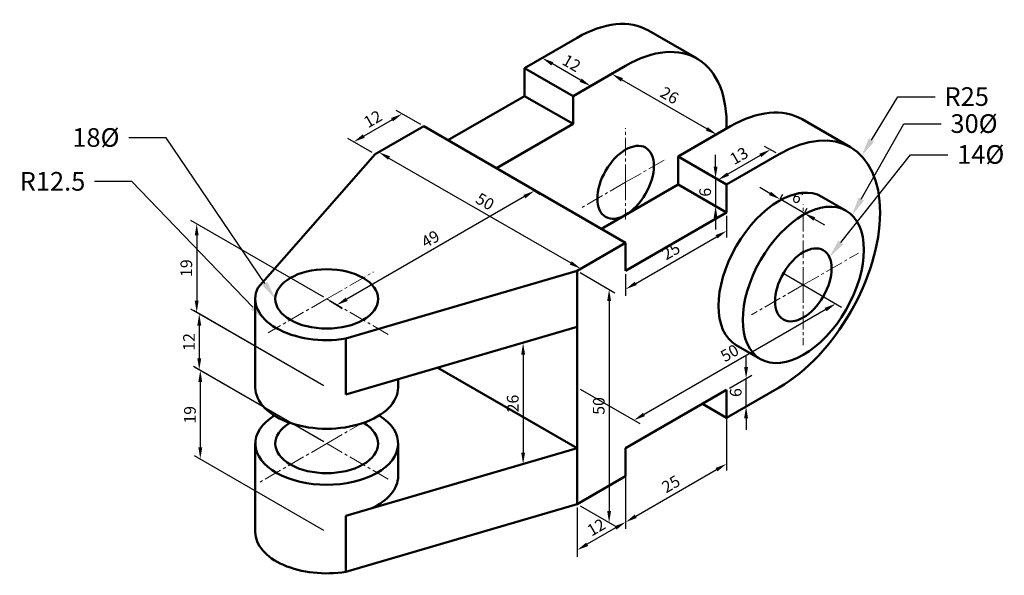
# Model space of a CAD drawing. Units: millimetres. Extents: x 313450 to 313661, y 30813 to 30932.
import ezdxf
from ezdxf import colors
from ezdxf.entities.mleader import LeaderData, LeaderLine
from ezdxf.math import Vec2, Vec3

# ---------------------------------------------------------------- set-up
doc = ezdxf.new("R2010")
doc.units = ezdxf.units.MM
doc.linetypes.add('CENTER2', pattern=[28.575, 19.05, -3.175, 3.175, -3.175])
for name, color, linetype, lineweight in [('M-CNTR', 1, 'CENTER2', 18), ('M-DIMS', 2, 'Continuous', 25), ('M-OUTL', 7, 'Continuous', 50), ('M-TEXT', 3, 'Continuous', 25)]:
    doc.layers.add(name, color=color, linetype=linetype, lineweight=lineweight)
doc.styles.get("Standard").update_dxf_attribs({"font": 'arial.ttf'})
doc.dimstyles.new('ISO-25', dxfattribs={"dimtxt": 2.5, "dimasz": 2.5, "dimexe": 1.25, "dimexo": 0.625, "dimtad": 1, "dimtxsty": 'Standard', "dimcen": 2.5, "dimadec": 0, "dimazin": 0, "dimtfac": 1, "dimtmove": 0, "dimatfit": 3, "dimfxl": 1, "dimarcsym": 0})

# ---------------------------------------------------------------- blocks, each defined once
blk = doc.blocks.new('*D1')
at = {"layer": 'Defpoints', "color": 0, "transparency": 16777216}
for p in [(313579.56, 30834.63), (313569.17, 30828.63), (313569.17, 30818.78)]:
    blk.add_point(p, dxfattribs=at)
at = {"layer": 'M-DIMS', "color": 0, "lineweight": -2, "transparency": 16777216}
for p, q in [((313579.56, 30833.91), (313579.56, 30823.33)), ((313569.17, 30827.91), (313569.17, 30817.33)), ((313577.39, 30823.53), (313571.33, 30820.03))]:
    blk.add_line(p, q, dxfattribs=at)
at = {"layer": 'M-DIMS', "color": 0, "transparency": 16777216}
for points in [[(313577.18, 30823.89), (313577.6, 30823.16), (313579.56, 30824.78)], [(313571.12, 30820.39), (313571.54, 30819.66), (313569.17, 30818.78)]]:
    blk.add_solid(points, dxfattribs=at)
at = {"layer": 'M-DIMS', "color": 0, "transparency": 16777216, "insert": (313573.42, 30823.4), "char_height": 2.5, "attachment_point": 5, "rotation": 30}
blk.add_mtext('12', dxfattribs=at)
blk = doc.blocks.new('*D2')
at = {"layer": 'Defpoints', "color": 0, "transparency": 16777216}
for p in [(313601.21, 30853.13), (313579.56, 30840.63), (313601.21, 30837.28)]:
    blk.add_point(p, dxfattribs=at)
at = {"layer": 'M-DIMS', "color": 0, "lineweight": -2, "transparency": 16777216}
for p, q in [((313601.21, 30852.41), (313601.21, 30835.83)), ((313579.56, 30839.91), (313579.56, 30823.33)), ((313581.72, 30826.03), (313599.04, 30836.03))]:
    blk.add_line(p, q, dxfattribs=at)
at = {"layer": 'M-DIMS', "color": 0, "transparency": 16777216}
for points in [[(313598.84, 30836.39), (313599.25, 30835.66), (313601.21, 30837.28)], [(313581.51, 30826.39), (313581.93, 30825.66), (313579.56, 30824.78)]]:
    blk.add_solid(points, dxfattribs=at)
at = {"layer": 'M-DIMS', "color": 0, "transparency": 16777216, "insert": (313589.43, 30832.67), "char_height": 2.5, "attachment_point": 5, "rotation": 30}
blk.add_mtext('25', dxfattribs=at)
blk = doc.blocks.new('*D3')
at = {"layer": 'Defpoints', "color": 0, "transparency": 16777216}
for p in [(313605.39, 30855.55), (313601.21, 30853.13), (313601.21, 30847.13)]:
    blk.add_point(p, dxfattribs=at)
at = {"layer": 'M-DIMS', "color": 0, "lineweight": -2, "transparency": 16777216}
for p, q in [((313605.39, 30858.05), (313605.39, 30860.55)), ((313601.83, 30853.49), (313606.64, 30856.27)), ((313605.39, 30849.55), (313605.39, 30855.55)), ((313601.83, 30847.49), (313606.64, 30850.27)), ((313605.39, 30847.05), (313605.39, 30844.55))]:
    blk.add_line(p, q, dxfattribs=at)
at = {"layer": 'M-DIMS', "color": 0, "transparency": 16777216}
for points in [[(313604.97, 30858.05), (313605.81, 30858.05), (313605.39, 30855.55)], [(313604.97, 30847.05), (313605.81, 30847.05), (313605.39, 30849.55)]]:
    blk.add_solid(points, dxfattribs=at)
at = {"layer": 'M-DIMS', "color": 0, "transparency": 16777216, "insert": (313603.49, 30852.55), "char_height": 2.5, "attachment_point": 5, "rotation": 90}
blk.add_mtext('6', dxfattribs=at)
blk = doc.blocks.new('*D4')
at = {"layer": 'Defpoints', "color": 0, "transparency": 16777216}
for p in [(313569.17, 30878.63), (313569.17, 30828.63), (313576.02, 30824.68)]:
    blk.add_point(p, dxfattribs=at)
at = {"layer": 'M-DIMS', "color": 0, "lineweight": -2, "transparency": 16777216}
for p, q in [((313569.79, 30878.27), (313577.27, 30873.95)), ((313576.02, 30872.18), (313576.02, 30827.18)), ((313569.79, 30828.27), (313577.27, 30823.95))]:
    blk.add_line(p, q, dxfattribs=at)
at = {"layer": 'M-DIMS', "color": 0, "transparency": 16777216}
for points in [[(313575.6, 30872.18), (313576.44, 30872.18), (313576.02, 30874.68)], [(313575.6, 30827.18), (313576.44, 30827.18), (313576.02, 30824.68)]]:
    blk.add_solid(points, dxfattribs=at)
at = {"layer": 'M-DIMS', "color": 0, "transparency": 16777216, "insert": (313574.12, 30849.68), "char_height": 2.5, "attachment_point": 5, "rotation": 90}
blk.add_mtext('50', dxfattribs=at)
blk = doc.blocks.new('*D5')
at = {"layer": 'Defpoints', "color": 0, "transparency": 16777216}
for p in [(313601.21, 30891.13), (313601.21, 30887.21), (313579.56, 30878.63)]:
    blk.add_point(p, dxfattribs=at)
at = {"layer": 'M-DIMS', "color": 0, "lineweight": -2, "transparency": 16777216}
for p, q in [((313601.21, 30890.41), (313601.21, 30885.77)), ((313581.72, 30875.96), (313599.04, 30885.96)), ((313579.56, 30877.91), (313579.56, 30873.27))]:
    blk.add_line(p, q, dxfattribs=at)
at = {"layer": 'M-DIMS', "color": 0, "transparency": 16777216}
for points in [[(313598.84, 30886.32), (313599.25, 30885.6), (313601.21, 30887.21)], [(313581.51, 30876.32), (313581.93, 30875.6), (313579.56, 30874.71)]]:
    blk.add_solid(points, dxfattribs=at)
at = {"layer": 'M-DIMS', "color": 0, "transparency": 16777216, "insert": (313589.43, 30882.61), "char_height": 2.5, "attachment_point": 5, "rotation": 30}
blk.add_mtext('25', dxfattribs=at)
blk = doc.blocks.new('*D6')
at = {"layer": 'Defpoints', "color": 0, "transparency": 16777216}
for p in [(313601.21, 30897.13), (313598.85, 30892.5), (313601.21, 30891.13)]:
    blk.add_point(p, dxfattribs=at)
at = {"layer": 'M-DIMS', "color": 0, "lineweight": -2, "transparency": 16777216}
for p, q in [((313598.85, 30901), (313598.85, 30903.5)), ((313600.58, 30897.49), (313597.6, 30899.22)), ((313598.85, 30898.5), (313598.85, 30892.5)), ((313600.58, 30891.49), (313597.6, 30893.22)), ((313598.85, 30890), (313598.85, 30887.5))]:
    blk.add_line(p, q, dxfattribs=at)
at = {"layer": 'M-DIMS', "color": 0, "transparency": 16777216}
for points in [[(313598.43, 30901), (313599.26, 30901), (313598.85, 30898.5)], [(313598.43, 30890), (313599.26, 30890), (313598.85, 30892.5)]]:
    blk.add_solid(points, dxfattribs=at)
at = {"layer": 'M-DIMS', "color": 0, "transparency": 16777216, "insert": (313596.94, 30895.5), "char_height": 2.5, "attachment_point": 5, "rotation": 90}
blk.add_mtext('6', dxfattribs=at)
blk = doc.blocks.new('*D7')
at = {"layer": 'Defpoints', "color": 0, "transparency": 16777216}
for p in [(313612.47, 30903.63), (313599.34, 30898.14), (313601.21, 30897.13)]:
    blk.add_point(p, dxfattribs=at)
at = {"layer": 'M-DIMS', "color": 0, "lineweight": -2, "transparency": 16777216}
for p, q in [((313608.44, 30903.39), (313601.51, 30899.39)), ((313611.82, 30903.98), (313609.31, 30905.34)), ((313600.56, 30897.48), (313598.05, 30898.84))]:
    blk.add_line(p, q, dxfattribs=at)
at = {"layer": 'M-DIMS', "color": 0, "transparency": 16777216}
for points in [[(313608.23, 30903.75), (313608.64, 30903.03), (313610.6, 30904.64)], [(313601.3, 30899.75), (313601.72, 30899.03), (313599.34, 30898.14)]]:
    blk.add_solid(points, dxfattribs=at)
at = {"layer": 'M-DIMS', "color": 0, "transparency": 16777216, "insert": (313604.02, 30903.04), "char_height": 2.5, "attachment_point": 5, "rotation": 30}
blk.add_mtext('13', dxfattribs=at)
blk = doc.blocks.new('*D8')
at = {"layer": 'Defpoints', "color": 0, "transparency": 16777216}
for p in [(313612.47, 30893.63), (313612.68, 30894), (313617.66, 30890.63)]:
    blk.add_point(p, dxfattribs=at)
at = {"layer": 'M-DIMS', "color": 0, "lineweight": -2, "transparency": 16777216}
for p, q in [((313610.51, 30895.25), (313608.35, 30896.5)), ((313612.78, 30894.17), (313613.3, 30895.08)), ((313617.87, 30891), (313612.68, 30894)), ((313617.98, 30891.17), (313618.5, 30892.08)), ((313620.04, 30889.75), (313622.2, 30888.5))]:
    blk.add_line(p, q, dxfattribs=at)
at = {"layer": 'M-DIMS', "color": 0, "transparency": 16777216}
for points in [[(313610.72, 30895.61), (313610.3, 30894.89), (313612.68, 30894)], [(313620.25, 30890.11), (313619.83, 30889.39), (313617.87, 30891)]]:
    blk.add_solid(points, dxfattribs=at)
at = {"layer": 'M-DIMS', "color": 0, "transparency": 16777216, "insert": (313616.23, 30894.14), "char_height": 2.5, "attachment_point": 5, "rotation": 330}
blk.add_mtext('6', dxfattribs=at)
blk = doc.blocks.new('*D9')
at = {"layer": 'Defpoints', "color": 0, "transparency": 16777216}
for p in [(313612.47, 30878.63), (313569.17, 30853.63), (313581.33, 30846.61)]:
    blk.add_point(p, dxfattribs=at)
at = {"layer": 'M-DIMS', "color": 0, "lineweight": -2, "transparency": 16777216}
for p, q in [((313613.09, 30878.27), (313625.88, 30870.89)), ((313622.47, 30870.36), (313583.5, 30847.86)), ((313569.79, 30853.27), (313582.58, 30845.89))]:
    blk.add_line(p, q, dxfattribs=at)
at = {"layer": 'M-DIMS', "color": 0, "transparency": 16777216}
for points in [[(313622.26, 30870.72), (313622.67, 30870), (313624.63, 30871.61)], [(313583.29, 30848.22), (313583.7, 30847.5), (313581.33, 30846.61)]]:
    blk.add_solid(points, dxfattribs=at)
at = {"layer": 'M-DIMS', "color": 0, "transparency": 16777216, "insert": (313602.03, 30860.76), "char_height": 2.5, "attachment_point": 5, "rotation": 30}
blk.add_mtext('50', dxfattribs=at)
blk = doc.blocks.new('*D10')
at = {"layer": 'Defpoints', "color": 0, "transparency": 16777216}
for p in [(313576.61, 30920.85), (313568.3, 30916.13), (313590.82, 30903.13)]:
    blk.add_point(p, dxfattribs=at)
at = {"layer": 'M-DIMS', "color": 0, "lineweight": -2, "transparency": 16777216}
for p, q in [((313568.93, 30916.49), (313577.87, 30921.56)), ((313596.96, 30909.1), (313578.77, 30919.6)), ((313591.45, 30903.49), (313600.39, 30908.56))]:
    blk.add_line(p, q, dxfattribs=at)
at = {"layer": 'M-DIMS', "color": 0, "transparency": 16777216}
for points in [[(313578.98, 30919.96), (313578.56, 30919.23), (313576.61, 30920.85)], [(313597.17, 30909.46), (313596.75, 30908.73), (313599.12, 30907.85)]]:
    blk.add_solid(points, dxfattribs=at)
at = {"layer": 'M-DIMS', "color": 0, "transparency": 16777216, "insert": (313588.82, 30915.99), "char_height": 2.5, "attachment_point": 5, "rotation": 330}
blk.add_mtext('26', dxfattribs=at)
blk = doc.blocks.new('*D11')
at = {"layer": 'Defpoints', "color": 0, "transparency": 16777216}
for p in [(313561.68, 30924.27), (313557.91, 30922.13), (313568.3, 30916.13)]:
    blk.add_point(p, dxfattribs=at)
at = {"layer": 'M-DIMS', "color": 0, "lineweight": -2, "transparency": 16777216}
for p, q in [((313558.54, 30922.49), (313562.94, 30924.99)), ((313569.91, 30919.52), (313563.85, 30923.02)), ((313568.93, 30916.49), (313573.33, 30918.99))]:
    blk.add_line(p, q, dxfattribs=at)
at = {"layer": 'M-DIMS', "color": 0, "transparency": 16777216}
for points in [[(313564.05, 30923.38), (313563.64, 30922.66), (313561.68, 30924.27)], [(313570.12, 30919.88), (313569.7, 30919.16), (313572.07, 30918.27)]]:
    blk.add_solid(points, dxfattribs=at)
at = {"layer": 'M-DIMS', "color": 0, "transparency": 16777216, "insert": (313567.82, 30922.9), "char_height": 2.5, "attachment_point": 5, "rotation": 330}
blk.add_mtext('12', dxfattribs=at)
blk = doc.blocks.new('*D12')
at = {"layer": 'Defpoints', "color": 0, "transparency": 16777216}
for p in [(313536.26, 30909.63), (313579.56, 30884.63), (313569.96, 30879.09)]:
    blk.add_point(p, dxfattribs=at)
at = {"layer": 'M-DIMS', "color": 0, "lineweight": -2, "transparency": 16777216}
for p, q in [((313535.63, 30909.27), (313525.41, 30903.37)), ((313528.82, 30902.84), (313567.8, 30880.34)), ((313578.93, 30884.27), (313568.71, 30878.37))]:
    blk.add_line(p, q, dxfattribs=at)
at = {"layer": 'M-DIMS', "color": 0, "transparency": 16777216}
for points in [[(313529.03, 30903.2), (313528.62, 30902.48), (313526.66, 30904.09)], [(313568, 30880.7), (313567.59, 30879.98), (313569.96, 30879.09)]]:
    blk.add_solid(points, dxfattribs=at)
at = {"layer": 'M-DIMS', "color": 0, "transparency": 16777216, "insert": (313549.26, 30893.24), "char_height": 2.5, "attachment_point": 5, "rotation": 330}
blk.add_mtext('50', dxfattribs=at)
blk = doc.blocks.new('*D13')
at = {"layer": 'Defpoints', "color": 0, "transparency": 16777216}
for p in [(313557.91, 30897.13), (313515.47, 30872.63), (313517.59, 30871.31)]:
    blk.add_point(p, dxfattribs=at)
at = {"layer": 'M-DIMS', "color": 0, "lineweight": -2, "transparency": 16777216}
for p, q in [((313558.51, 30896.76), (313561.22, 30895.05)), ((313557.86, 30894.56), (313519.75, 30872.56)), ((313516.07, 30872.26), (313518.79, 30870.55))]:
    blk.add_line(p, q, dxfattribs=at)
at = {"layer": 'M-DIMS', "color": 0, "transparency": 16777216}
for points in [[(313557.65, 30894.92), (313558.07, 30894.19), (313560.02, 30895.81)], [(313519.55, 30872.92), (313519.96, 30872.19), (313517.59, 30871.31)]]:
    blk.add_solid(points, dxfattribs=at)
at = {"layer": 'M-DIMS', "color": 0, "transparency": 16777216, "insert": (313537.86, 30885.2), "char_height": 2.5, "attachment_point": 5, "rotation": 30}
blk.add_mtext('49', dxfattribs=at)
blk = doc.blocks.new('*D14')
at = {"layer": 'Defpoints', "color": 0, "transparency": 16777216}
for p in [(313536.26, 30909.63), (313521.25, 30906.3), (313525.86, 30903.63)]:
    blk.add_point(p, dxfattribs=at)
at = {"layer": 'M-DIMS', "color": 0, "lineweight": -2, "transparency": 16777216}
for p, q in [((313535.63, 30909.99), (313530.39, 30913.02)), ((313529.48, 30911.05), (313523.41, 30907.55)), ((313525.24, 30903.99), (313520, 30907.02))]:
    blk.add_line(p, q, dxfattribs=at)
at = {"layer": 'M-DIMS', "color": 0, "transparency": 16777216}
for points in [[(313529.27, 30911.41), (313529.68, 30910.69), (313531.64, 30912.3)], [(313523.21, 30907.91), (313523.62, 30907.19), (313521.25, 30906.3)]]:
    blk.add_solid(points, dxfattribs=at)
at = {"layer": 'M-DIMS', "color": 0, "transparency": 16777216, "insert": (313525.51, 30910.93), "char_height": 2.5, "attachment_point": 5, "rotation": 30}
blk.add_mtext('12', dxfattribs=at)
blk = doc.blocks.new('*D15')
at = {"layer": 'Defpoints', "color": 0, "transparency": 16777216}
for p in [(313515.47, 30872.63), (313487.59, 30869.73), (313515.47, 30853.63)]:
    blk.add_point(p, dxfattribs=at)
at = {"layer": 'M-DIMS', "color": 0, "lineweight": -2, "transparency": 16777216}
for p, q in [((313514.85, 30872.99), (313486.34, 30889.45)), ((313487.59, 30886.23), (313487.59, 30872.23)), ((313514.85, 30853.99), (313486.34, 30870.45))]:
    blk.add_line(p, q, dxfattribs=at)
at = {"layer": 'M-DIMS', "color": 0, "transparency": 16777216}
for points in [[(313487.17, 30886.23), (313488.01, 30886.23), (313487.59, 30888.73)], [(313487.17, 30872.23), (313488.01, 30872.23), (313487.59, 30869.73)]]:
    blk.add_solid(points, dxfattribs=at)
at = {"layer": 'M-DIMS', "color": 0, "transparency": 16777216, "insert": (313485.69, 30879.23), "char_height": 2.5, "attachment_point": 5, "rotation": 90}
blk.add_mtext('19', dxfattribs=at)
blk = doc.blocks.new('*D16')
at = {"layer": 'Defpoints', "color": 0, "transparency": 16777216}
for p in [(313488.14, 30857.41), (313515.47, 30853.63), (313515.47, 30841.63)]:
    blk.add_point(p, dxfattribs=at)
at = {"layer": 'M-DIMS', "color": 0, "lineweight": -2, "transparency": 16777216}
for p, q in [((313514.85, 30853.99), (313486.89, 30870.13)), ((313488.14, 30866.91), (313488.14, 30859.91)), ((313514.85, 30841.99), (313486.89, 30858.13))]:
    blk.add_line(p, q, dxfattribs=at)
at = {"layer": 'M-DIMS', "color": 0, "transparency": 16777216}
for points in [[(313487.72, 30866.91), (313488.56, 30866.91), (313488.14, 30869.41)], [(313487.72, 30859.91), (313488.56, 30859.91), (313488.14, 30857.41)]]:
    blk.add_solid(points, dxfattribs=at)
at = {"layer": 'M-DIMS', "color": 0, "transparency": 16777216, "insert": (313486.26, 30863.41), "char_height": 2.5, "attachment_point": 5, "rotation": 90}
blk.add_mtext('12', dxfattribs=at)
blk = doc.blocks.new('*D17')
at = {"layer": 'Defpoints', "color": 0, "transparency": 16777216}
for p in [(313515.47, 30841.63), (313488.36, 30838.29), (313515.47, 30822.63)]:
    blk.add_point(p, dxfattribs=at)
at = {"layer": 'M-DIMS', "color": 0, "lineweight": -2, "transparency": 16777216}
for p, q in [((313514.85, 30841.99), (313487.11, 30858.01)), ((313488.36, 30854.79), (313488.36, 30840.79)), ((313514.85, 30822.99), (313487.11, 30839.01))]:
    blk.add_line(p, q, dxfattribs=at)
at = {"layer": 'M-DIMS', "color": 0, "transparency": 16777216}
for points in [[(313487.94, 30854.79), (313488.78, 30854.79), (313488.36, 30857.29)], [(313487.94, 30840.79), (313488.78, 30840.79), (313488.36, 30838.29)]]:
    blk.add_solid(points, dxfattribs=at)
at = {"layer": 'M-DIMS', "color": 0, "transparency": 16777216, "insert": (313486.46, 30847.79), "char_height": 2.5, "attachment_point": 5, "rotation": 90}
blk.add_mtext('19', dxfattribs=at)
blk = doc.blocks.new('*D18')
at = {"layer": 'Defpoints', "color": 0, "transparency": 16777216}
for p in [(313569.17, 30866.63), (313569.17, 30840.63), (313557.58, 30837.2)]:
    blk.add_point(p, dxfattribs=at)
at = {"layer": 'M-DIMS', "color": 0, "lineweight": -2, "transparency": 16777216}
for p, q in [((313568.54, 30866.45), (313556.33, 30862.83)), ((313557.58, 30860.7), (313557.58, 30839.7)), ((313568.54, 30840.45), (313556.33, 30836.83))]:
    blk.add_line(p, q, dxfattribs=at)
at = {"layer": 'M-DIMS', "color": 0, "transparency": 16777216}
for points in [[(313557.17, 30860.7), (313558, 30860.7), (313557.58, 30863.2)], [(313557.17, 30839.7), (313558, 30839.7), (313557.58, 30837.2)]]:
    blk.add_solid(points, dxfattribs=at)
at = {"layer": 'M-DIMS', "color": 0, "transparency": 16777216, "insert": (313555.68, 30850.2), "char_height": 2.5, "attachment_point": 5, "rotation": 90}
blk.add_mtext('26', dxfattribs=at)

msp = doc.modelspace()

# ---------------------------------------------------------------- linework, layer by layer
at = {"layer": 'M-CNTR', "ltscale": 0.2}
for p, q in [((313579.558, 30897.633), (313579.558, 30909.221)), ((313579.558, 30897.633), (313588.285, 30902.671)), ((313579.558, 30897.633), (313570.042, 30892.139)), ((313579.558, 30897.633), (313579.558, 30889.642)), ((313617.663, 30875.633), (313617.663, 30892.9)), ((313617.663, 30875.633), (313629.477, 30882.454)), ((313515.472, 30872.633), (313525.465, 30878.402)), ((313617.663, 30875.633), (313606.535, 30869.208)), ((313617.663, 30875.633), (313617.663, 30862.712)), ((313617.663, 30875.633), (313617.663, 30875.633)), ((313515.472, 30872.633), (313502.891, 30865.369)), ((313515.472, 30872.633), (313528.832, 30864.919)), ((313515.472, 30841.633), (313522.437, 30845.654)), ((313515.472, 30841.633), (313501.156, 30833.367)), ((313515.472, 30841.633), (313529.129, 30833.748))]:
    msp.add_line(p, q, dxfattribs=at)
at = {"layer": 'M-OUTL'}
for p, q in [((313557.907, 30922.133), (313569.166, 30928.633)), ((313584.475, 30930.149), (313594.867, 30924.149)), ((313568.299, 30916.133), (313579.558, 30922.633)), ((313557.907, 30922.133), (313568.299, 30916.133)), ((313557.907, 30916.133), (313557.907, 30922.133)), ((313557.907, 30916.133), (313541.453, 30906.633)), ((313568.299, 30910.133), (313557.907, 30916.133)), ((313568.299, 30916.133), (313568.299, 30910.133)), ((313536.257, 30909.633), (313525.864, 30903.633)), ((313579.558, 30884.633), (313536.257, 30909.633)), ((313568.299, 30910.133), (313551.845, 30900.633)), ((313590.816, 30903.133), (313602.074, 30909.633)), ((313617.384, 30911.149), (313627.776, 30905.149)), ((313500.722, 30875), (313525.864, 30903.633)), ((313601.208, 30897.133), (313612.467, 30903.633)), ((313590.816, 30897.133), (313590.816, 30903.133)), ((313590.816, 30903.133), (313601.208, 30897.133)), ((313590.816, 30897.133), (313574.362, 30887.633)), ((313601.208, 30891.133), (313590.816, 30897.133)), ((313601.208, 30891.133), (313601.208, 30897.133)), ((313621.652, 30894.543), (313626.849, 30891.543)), ((313579.558, 30878.633), (313601.208, 30891.133)), ((313569.166, 30878.633), (313579.558, 30884.633)), ((313569.166, 30878.633), (313579.558, 30884.633)), ((313579.558, 30884.633), (313579.558, 30878.633)), ((313519.573, 30864.117), (313569.166, 30878.633)), ((313569.166, 30828.633), (313569.166, 30878.633)), ((313569.166, 30878.633), (313569.166, 30866.633)), ((313500.163, 30872.633), (313500.163, 30853.633)), ((313569.166, 30866.633), (313519.573, 30852.117)), ((313519.573, 30864.117), (313519.573, 30852.117)), ((313519.573, 30864.117), (313519.573, 30852.117)), ((313603.281, 30862.723), (313608.477, 30859.723)), ((313569.166, 30840.633), (313539.282, 30857.886)), ((313530.781, 30853.633), (313530.781, 30855.398)), ((313579.558, 30840.633), (313601.208, 30853.133)), ((313601.208, 30847.133), (313612.467, 30853.633)), ((313601.208, 30853.133), (313601.208, 30847.133)), ((313601.208, 30847.133), (313596.012, 30850.133)), ((313500.163, 30834.633), (313500.163, 30841.633)), ((313519.573, 30826.117), (313569.166, 30840.633)), ((313530.781, 30834.633), (313530.781, 30841.633)), ((313569.166, 30828.633), (313569.166, 30840.633)), ((313579.558, 30834.633), (313579.558, 30840.633)), ((313500.163, 30822.633), (313500.163, 30834.633)), ((313569.166, 30828.633), (313579.558, 30834.633)), ((313519.573, 30814.117), (313569.166, 30828.633)), ((313519.573, 30814.117), (313519.573, 30826.117)), ((313519.573, 30826.117), (313519.573, 30814.117))]:
    msp.add_line(p, q, dxfattribs=at)
for centre, major_axis, start_param, end_param in [((313569.166, 30903.633), (-15.309, -26.517), 9.424778, 10.2101761), ((313579.558, 30897.633), (-15.309, -26.517), 8.5993691, 10.2101761), ((313602.074, 30884.633), (-15.309, -26.517), 9.424778, 10.2101761), ((313612.467, 30878.633), (-15.309, -26.517), 0.7853982, 3.9269908), ((313612.467, 30878.633), (-9.186, -15.91), 3.1415927, 6.2831853), ((313515.472, 30872.633), (-15.309, 0), 6.0119996, 8.1251673), ((313515.472, 30853.633), (-15.309, 0), 0, 3.1415927), ((313515.472, 30841.633), (-15.309, 0), 5.5370274, 10.1709359), ((313515.472, 30841.633), (-11.023, 0), 5.5127225, 10.1952408), ((313515.472, 30834.633), (-15.309, 0), 8.521217, 9.424778), ((313515.472, 30822.633), (-15.309, 0), 6.2831853, 8.1251673)]:
    msp.add_ellipse(centre, major_axis=major_axis, ratio=0.5773503, start_param=start_param, end_param=end_param, dxfattribs=at)
for centre, major_axis in [((313579.558, 30897.633), (-4.287, -7.425)), ((313617.663, 30875.633), (-9.186, -15.91)), ((313617.663, 30875.633), (-4.287, -7.425)), ((313515.472, 30872.633), (-11.023, 0))]:
    msp.add_ellipse(centre, major_axis=major_axis, ratio=0.5773503, dxfattribs=at)

# ---------------------------------------------------------------- dimensions: what is measured, and where the dimension line sits
at = {"layer": 'M-DIMS'}
for p1, p2, distance, picture, middle in [((313568.299, 30916.133), (313557.907, 30922.133), -3.741, '*D11', (313567.817, 30922.902)), ((313590.816, 30903.133), (313568.299, 30916.133), -8.235, '*D10', (313588.816, 30915.992)), ((313536.257, 30909.633), (313525.864, 30903.633), -4.615, '*D14', (313525.505, 30910.925)), ((313536.257, 30909.633), (313579.558, 30884.633), -9.597, '*D12', (313549.261, 30893.238)), ((313612.467, 30903.633), (313601.208, 30897.133), -1.809, '*D7', (313604.02, 30903.041)), ((313601.208, 30897.133), (313601.208, 30891.133), -2.362, '*D6', (313596.945, 30895.496)), ((313557.907, 30897.133), (313515.472, 30872.633), 2.208, '*D13', (313537.856, 30885.202)), ((313617.663, 30890.633), (313612.467, 30893.633), -0.42, '*D8', (313616.226, 30894.143)), ((313579.558, 30878.633), (313601.208, 30891.133), -3.394, '*D5', (313589.432, 30882.61)), ((313515.472, 30872.633), (313515.472, 30853.633), -27.883, '*D15', (313485.687, 30879.231)), ((313569.166, 30878.633), (313569.166, 30828.633), 6.853, '*D4', (313574.118, 30849.676)), ((313612.467, 30878.633), (313569.166, 30853.633), 12.165, '*D9', (313602.03, 30860.756)), ((313515.472, 30853.633), (313515.472, 30841.633), -27.333, '*D16', (313486.259, 30863.413)), ((313569.166, 30866.633), (313569.166, 30840.633), -11.582, '*D18', (313555.683, 30850.199)), ((313601.208, 30847.133), (313601.208, 30853.133), -4.183, '*D3', (313603.49, 30852.548)), ((313515.472, 30841.633), (313515.472, 30822.633), -27.111, '*D17', (313486.459, 30847.785)), ((313579.558, 30840.633), (313601.208, 30853.133), -13.733, '*D2', (313589.432, 30832.672)), ((313579.558, 30834.633), (313569.166, 30828.633), 8.537, '*D1', (313573.422, 30823.403))]:
    dim = msp.add_aligned_dim(p1=p1, p2=p2, distance=distance, dimstyle='ISO-25', override={"dimclrd": 0, "dimclre": 0, "dimclrt": 0}, dxfattribs=at)
    dim.commit()
    dim.dimension.update_dxf_attribs({"geometry": picture, "text_midpoint": middle})

# ---------------------------------------------------------------- leaders
at = {"layer": 'M-TEXT'}
ml = msp.add_multileader_mtext('Standard', dxfattribs=at)
ml.set_content('R25', color=256)
ml.set_leader_properties()
ml.build(insert=Vec2(0, 0))
ctx = ml.context
ctx.base_point, ctx.plane_origin = Vec3(313645.933, 30915.982), Vec3(313630.16, 30903.256)
notes = []
notes.append((ctx, [(0, (1, 1, 0), (313637.933, 30915.982), (1, 0), 8, [(0, [(313630.16, 30903.256)], 0, [])])]))
ctx.mtext.insert, ctx.mtext.flow_direction = Vec3(313647.933, 30918.016), 5
ml = msp.add_multileader_mtext('Standard', dxfattribs=at)
ml.set_content('30%%C', color=256)
ml.set_leader_properties()
ml.build(insert=Vec2(0, 0))
ctx = ml.context
ctx.base_point, ctx.plane_origin = Vec3(313647.205, 30910.142), Vec3(313628.121, 30890.568)
notes.append((ctx, [(0, (1, 1, 0), (313639.205, 30910.142), (1, 0), 8, [(0, [(313628.121, 30890.568)], 0, [])])]))
ctx.mtext.insert, ctx.mtext.flow_direction = Vec3(313649.205, 30912.223), 5
ml = msp.add_multileader_mtext('Standard', dxfattribs=at)
ml.set_content('18%%C', color=256)
ml.set_leader_properties()
ml.build(insert=Vec2(0, 0))
ctx = ml.context
ctx.base_point, ctx.plane_origin = Vec3(313459.28, 30907.162), Vec3(313504.449, 30872.633)
ctx.text_align_type = 2
notes.append((ctx, [(0, (1, 1, 0), (313481.026, 30907.162), (-1, 0), 8, [(0, [(313504.449, 30872.633)], 0, [])])]))
ctx.mtext.insert, ctx.mtext.alignment, ctx.mtext.flow_direction = Vec3(313471.026, 30909.242), 3, 5
ml = msp.add_multileader_mtext('Standard', dxfattribs=at)
ml.set_content('14%%C', color=256)
ml.set_leader_properties()
ml.build(insert=Vec2(0, 0))
ctx = ml.context
ctx.base_point, ctx.plane_origin = Vec3(313648.649, 30903.523), Vec3(313623.238, 30881.6)
notes.append((ctx, [(0, (1, 1, 0), (313640.649, 30903.523), (1, 0), 8, [(0, [(313623.238, 30881.6)], 0, [])])]))
ctx.mtext.insert, ctx.mtext.flow_direction = Vec3(313650.649, 30905.603), 5
ml = msp.add_multileader_mtext('Standard', dxfattribs=at)
ml.set_content('R12.5', color=256)
ml.set_leader_properties()
ml.build(insert=Vec2(0, 0))
ctx = ml.context
ctx.base_point, ctx.plane_origin = Vec3(313447.458, 30897.806), Vec3(313502.429, 30868.004)
ctx.text_align_type = 2
notes.append((ctx, [(0, (1, 1, 0), (313473.707, 30897.806), (-1, 0), 8, [(0, [(313502.429, 30868.004)], 0, [])])]))
ctx.mtext.insert, ctx.mtext.alignment, ctx.mtext.flow_direction = Vec3(313463.707, 30899.841), 3, 5
for ctx, leaders in notes:
    for number, flags, end, landing, length, lines in leaders:
        leader = LeaderData()
        leader.index, (leader.has_last_leader_line, leader.has_dogleg_vector, leader.attachment_direction) = number, flags
        leader.last_leader_point, leader.dogleg_vector, leader.dogleg_length = Vec3(end), Vec3(landing), length
        for number, points, colour, breaks in lines:
            line = LeaderLine()
            line.index, line.vertices, line.color, line.breaks = number, Vec3.list(points), colors.encode_raw_color(colour), breaks
            leader.lines.append(line)
        ctx.leaders.append(leader)

doc.saveas('drawing.dxf')
